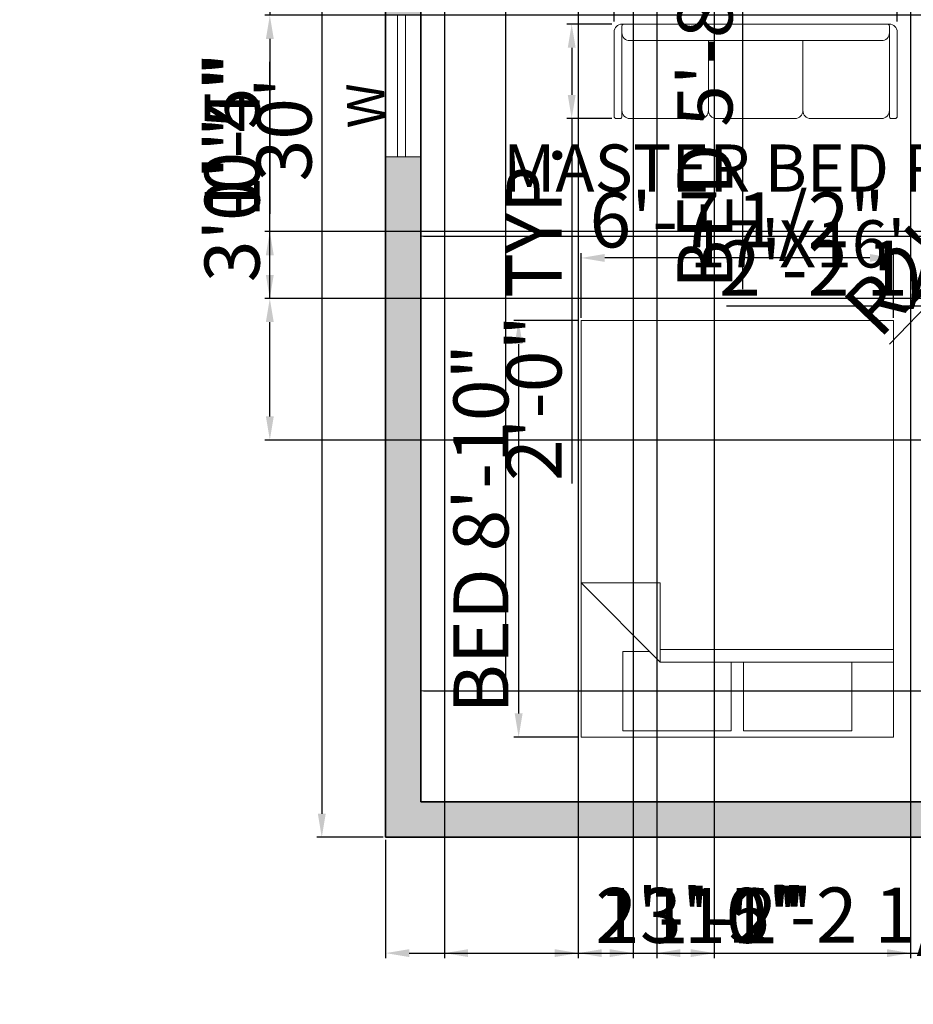
# Model space of a CAD drawing. Units: inches. Extents: x 2961 to 3748, y 1432 to 1961.
# Tile 1 of 9: x 2961 to 3188, y 1462 to 1713. Entities that reach past the tile are written whole.
import ezdxf
from ezdxf.enums import TextEntityAlignment as Align

# ---------------------------------------------------------------- set-up
doc = ezdxf.new("R2010")
doc.units = ezdxf.units.IN
for name, color, linetype, lineweight in [('A-ANNO-DIMS', 2, 'Continuous', 18), ('A-ANNO-TEXT', 7, 'Continuous', 18), ('A-AREA-IDEN', 7, 'Continuous', 18), ('A-FURN', 8, 'Continuous', 18), ('A-FURN-FIXD', 9, 'Continuous', 20), ('A-GLAZ', 4, 'Continuous', 18), ('A-WALL', 7, 'Continuous', 35), ('A-WALL-PATT', 252, 'Continuous', 13)]:
    doc.layers.add(name, color=color, linetype=linetype, lineweight=lineweight)
doc.styles.get("Standard").update_dxf_attribs({"font": 'arial.ttf'})
doc.dimstyles.new('ISO-25', dxfattribs={"dimtxt": 14, "dimasz": 6, "dimexe": 1.25, "dimexo": 0.625, "dimtad": 1, "dimlunit": 3, "dimtxsty": 'Standard', "dimcen": 2.5, "dimadec": 0, "dimazin": 0, "dimtfac": 1, "dimtmove": 0, "dimatfit": 3, "dimfxl": 1, "dimarcsym": 0})

# ---------------------------------------------------------------- blocks, each defined once
blk = doc.blocks.new('Bed - Queen')
for p, q in [((0, -80.00003), (0, 0)), ((0, 0), (59.99999, 0)), ((59.99999, 0), (59.99999, -80.00003)), ((7.99999, -1.2), (28.79998, -1.2)), ((7.99999, -14.4), (7.99999, -1.2)), ((28.79998, -1.2), (28.79998, -14.4)), ((31.19999, -1.2), (51.99999, -1.2)), ((31.19999, -14.4), (31.19999, -1.2)), ((51.99999, -1.2), (51.99999, -16.4)), ((0, -14.4), (44.8, -14.4)), ((59.99999, -29.6), (44.8, -14.4)), ((44.8, -14.4), (44.8, -29.6)), ((44.8, -16.8), (0, -16.8)), ((51.99999, -16.4), (46.79936, -16.4)), ((44.8, -29.6), (59.99999, -29.6)), ((59.99999, -80.00003), (0, -80.00003))]:
    blk.add_line(p, q)
blk = doc.blocks.new('sofa')
for p, q in [((1024.17, 311.16), (1024.17, 289.66)), ((1024.67, 311.66), (1025.67, 311.66)), ((1026.17, 308), (1026.17, 311.16)), ((1050.17, 311.66), (1070.17, 311.66)), ((1094.17, 309.66), (1094.17, 311.16)), ((1095.67, 311.66), (1094.67, 311.66)), ((1096.17, 289.66), (1096.17, 311.16)), ((1048.17, 309.66), (1048.17, 291.87)), ((1048.17, 309.66), (1048.17, 309.66)), ((1072.17, 309.66), (1072.17, 291.87)), ((1072.17, 309.66), (1072.17, 309.66)), ((1026.17, 287.66), (1094.17, 287.66))]:
    blk.add_line(p, q)
for points in [[(1046.17, 311.66), (1028.17, 311.66, 0.414214), (1026.17, 309.66), (1026.17, 288.16)], [(1074.17, 311.66), (1092.17, 311.66, -0.414214), (1094.17, 309.66), (1094.17, 288.16)]]:
    blk.add_lwpolyline(points, format="xyb")
blk.add_lwpolyline([(1026.67, 287.66), (1093.67, 287.66, 0.414214), (1094.17, 288.16), (1094.17, 289.87, 0.414214), (1092.17, 291.87), (1028.17, 291.87, 0.414214), (1026.17, 289.87), (1026.17, 288.16, 0.414214)], format="xyb", close=True)
for centre, radius, start, end in [((1024.67, 311.16), 0.5, 90, 180), ((1025.67, 311.16), 0.5, 0, 90), ((1046.17, 309.66), 2, 0, 90), ((1050.17, 309.66), 2, 90, 180), ((1070.17, 309.66), 2, 0, 90), ((1074.17, 309.66), 2, 90, 180), ((1094.67, 311.16), 0.5, 90, 180), ((1095.67, 311.16), 0.5, 0, 90), ((1026.17, 289.66), 2, 180, 270), ((1094.17, 289.66), 2, 270, 0)]:
    blk.add_arc(centre, radius, start, end)
blk = doc.blocks.new('*D15')
at = {"layer": 'A-ANNO-DIMS', "color": 0, "lineweight": -2, "transparency": 16777216}
for p, q in [((3053.64, 1864.64), (3036.79, 1864.64)), ((3038.04, 1858.64), (3038.04, 1510.64)), ((3053.64, 1504.64), (3036.79, 1504.64))]:
    blk.add_line(p, q, dxfattribs=at)
at = {"layer": 'A-ANNO-DIMS', "color": 0, "transparency": 16777216}
for points in [[(3037.04, 1858.64), (3039.04, 1858.64), (3038.04, 1864.64)], [(3037.04, 1510.64), (3039.04, 1510.64), (3038.04, 1504.64)]]:
    blk.add_solid(points, dxfattribs=at)
at = {"layer": 'Defpoints', "color": 0, "transparency": 16777216}
for p in [(3054.27, 1864.64), (3038.04, 1504.64), (3054.27, 1504.64)]:
    blk.add_point(p, dxfattribs=at)
at = {"layer": 'A-ANNO-DIMS', "color": 0, "transparency": 16777216, "insert": (3030.26, 1684.64), "char_height": 14, "attachment_point": 5, "rotation": 90}
blk.add_mtext("30'", dxfattribs=at)
blk = doc.blocks.new('WIN-36IN')
for p, q in [((0, 6), (36, 6)), ((0, 3.9), (36, 3.9))]:
    blk.add_line(p, q)
blk.add_lwpolyline([(36, 9), (0, 9), (0, 0), (36, 0)], close=True)
blk = doc.blocks.new('*D22')
at = {"layer": 'A-ANNO-DIMS', "color": 0, "lineweight": -2, "transparency": 16777216}
for p, q in [((3103.38, 1636.05), (3086.86, 1636.05)), ((3088.11, 1630.05), (3088.11, 1536.12)), ((3103.38, 1530.12), (3086.86, 1530.12))]:
    blk.add_line(p, q, dxfattribs=at)
at = {"layer": 'A-ANNO-DIMS', "color": 0, "transparency": 16777216}
for points in [[(3087.11, 1630.05), (3089.11, 1630.05), (3088.11, 1636.05)], [(3087.11, 1536.12), (3089.11, 1536.12), (3088.11, 1530.12)]]:
    blk.add_solid(points, dxfattribs=at)
at = {"layer": 'Defpoints', "color": 0, "transparency": 16777216}
for p in [(3104, 1636.05), (3088.11, 1530.12), (3104, 1530.12)]:
    blk.add_point(p, dxfattribs=at)
at = {"layer": 'A-ANNO-DIMS', "color": 0, "transparency": 16777216, "insert": (3080.34, 1583.09), "char_height": 14, "attachment_point": 5, "rotation": 90}
blk.add_mtext('BED 8\'-10"', dxfattribs=at)
blk = doc.blocks.new('*D23')
at = {"layer": 'A-ANNO-DIMS', "color": 0, "lineweight": -2, "transparency": 16777216}
for p, q in [((3104, 1636.67), (3104, 1653.19)), ((3183.44, 1636.67), (3183.44, 1653.19)), ((3177.44, 1651.94), (3110, 1651.94))]:
    blk.add_line(p, q, dxfattribs=at)
at = {"layer": 'A-ANNO-DIMS', "color": 0, "transparency": 16777216}
for points in [[(3110, 1652.94), (3110, 1650.94), (3104, 1651.94)], [(3177.44, 1652.94), (3177.44, 1650.94), (3183.44, 1651.94)]]:
    blk.add_solid(points, dxfattribs=at)
at = {"layer": 'Defpoints', "color": 0, "transparency": 16777216}
for p in [(3104, 1651.94), (3104, 1636.05), (3183.44, 1636.05)]:
    blk.add_point(p, dxfattribs=at)
at = {"layer": 'A-ANNO-DIMS', "color": 0, "transparency": 16777216, "insert": (3143.72, 1659.8), "char_height": 14, "attachment_point": 5}
blk.add_mtext('6\'-7 1/2"', dxfattribs=at)
blk = doc.blocks.new('*D24')
at = {"layer": 'A-ANNO-DIMS', "color": 0, "lineweight": -2, "transparency": 16777216}
for p, q in [((3154.63, 1801.29), (3143.84, 1801.29)), ((3145.09, 1795.29), (3145.09, 1739.5)), ((3154.63, 1733.5), (3143.84, 1733.5)), ((3145.09, 1733.5), (3145.09, 1644.01))]:
    blk.add_line(p, q, dxfattribs=at)
at = {"layer": 'A-ANNO-DIMS', "color": 0, "transparency": 16777216}
for points in [[(3144.09, 1795.29), (3146.09, 1795.29), (3145.09, 1801.29)], [(3144.09, 1739.5), (3146.09, 1739.5), (3145.09, 1733.5)]]:
    blk.add_solid(points, dxfattribs=at)
at = {"layer": 'Defpoints', "color": 0, "transparency": 16777216}
for p in [(3155.26, 1801.29), (3145.09, 1733.5), (3155.26, 1733.5)]:
    blk.add_point(p, dxfattribs=at)
at = {"layer": 'A-ANNO-DIMS', "color": 0, "transparency": 16777216, "insert": (3137.32, 1685.76), "char_height": 14, "attachment_point": 5, "rotation": 90}
blk.add_mtext('BED 5\'-8"', dxfattribs=at)
blk = doc.blocks.new('*D26')
at = {"layer": 'A-ANNO-DIMS', "color": 0, "lineweight": -2, "transparency": 16777216}
for p, q in [((3112.4, 1712.02), (3112.4, 1723.44)), ((3184.4, 1712.02), (3184.4, 1723.44)), ((3112.4, 1722.19), (2961.2, 1722.19)), ((3178.4, 1722.19), (3118.4, 1722.19))]:
    blk.add_line(p, q, dxfattribs=at)
at = {"layer": 'A-ANNO-DIMS', "color": 0, "transparency": 16777216}
for points in [[(3118.4, 1723.19), (3118.4, 1721.19), (3112.4, 1722.19)], [(3178.4, 1723.19), (3178.4, 1721.19), (3184.4, 1722.19)]]:
    blk.add_solid(points, dxfattribs=at)
at = {"layer": 'Defpoints', "color": 0, "transparency": 16777216}
for p in [(3112.4, 1722.19), (3112.4, 1711.39), (3184.4, 1711.39)]:
    blk.add_point(p, dxfattribs=at)
at = {"layer": 'A-ANNO-DIMS', "color": 0, "transparency": 16777216, "insert": (3033.8, 1730.06), "char_height": 14, "attachment_point": 5}
blk.add_mtext('SOFA 6\'-0" TYP.', dxfattribs=at)
blk = doc.blocks.new('*D27')
at = {"layer": 'A-ANNO-DIMS', "color": 0, "lineweight": -2, "transparency": 16777216}
for p, q in [((3111.78, 1711.39), (3100.35, 1711.39)), ((3101.6, 1705.39), (3101.6, 1693.39)), ((3111.78, 1687.39), (3100.35, 1687.39)), ((3101.6, 1687.39), (3101.6, 1594.57))]:
    blk.add_line(p, q, dxfattribs=at)
at = {"layer": 'A-ANNO-DIMS', "color": 0, "transparency": 16777216}
for points in [[(3100.6, 1705.39), (3102.6, 1705.39), (3101.6, 1711.39)], [(3100.6, 1693.39), (3102.6, 1693.39), (3101.6, 1687.39)]]:
    blk.add_solid(points, dxfattribs=at)
at = {"layer": 'Defpoints', "color": 0, "transparency": 16777216}
for p in [(3112.4, 1711.39), (3101.6, 1687.39), (3112.4, 1687.39)]:
    blk.add_point(p, dxfattribs=at)
at = {"layer": 'A-ANNO-DIMS', "color": 0, "transparency": 16777216, "insert": (3093.83, 1637.98), "char_height": 14, "attachment_point": 5, "rotation": 90}
blk.add_mtext('2\'-0" TYP.', dxfattribs=at)
blk = doc.blocks.new('*D29')
at = {"layer": 'A-ANNO-DIMS', "color": 0, "lineweight": -2, "transparency": 16777216}
for p, q in [((3218.32, 1632.29), (3218.32, 1640.93)), ((3245.04, 1632.29), (3245.04, 1640.93)), ((3218.32, 1639.68), (3140.99, 1639.68)), ((3239.04, 1639.68), (3224.32, 1639.68))]:
    blk.add_line(p, q, dxfattribs=at)
at = {"layer": 'A-ANNO-DIMS', "color": 0, "transparency": 16777216}
for points in [[(3224.32, 1640.68), (3224.32, 1638.68), (3218.32, 1639.68)], [(3239.04, 1640.68), (3239.04, 1638.68), (3245.04, 1639.68)]]:
    blk.add_solid(points, dxfattribs=at)
at = {"layer": 'Defpoints', "color": 0, "transparency": 16777216}
for p in [(3218.32, 1639.68), (3218.32, 1631.67), (3245.04, 1631.67)]:
    blk.add_point(p, dxfattribs=at)
at = {"layer": 'A-ANNO-DIMS', "color": 0, "transparency": 16777216, "insert": (3176.66, 1647.55), "char_height": 14, "attachment_point": 5}
blk.add_mtext('2\'-2 1/2"', dxfattribs=at)
blk = doc.blocks.new('*D53')
at = {"layer": 'A-ANNO-DIMS', "color": 0, "lineweight": -2, "transparency": 16777216}
for p, q in [((3123.27, 1855.01), (3123.27, 1473.94)), ((3187.8, 1855.01), (3187.8, 1473.94)), ((3129.27, 1475.19), (3181.8, 1475.19)), ((3187.8, 1475.19), (3264.89, 1475.19))]:
    blk.add_line(p, q, dxfattribs=at)
at = {"layer": 'A-ANNO-DIMS', "color": 0, "transparency": 16777216}
for points in [[(3129.27, 1476.19), (3129.27, 1474.19), (3123.27, 1475.19)], [(3181.8, 1476.19), (3181.8, 1474.19), (3187.8, 1475.19)]]:
    blk.add_solid(points, dxfattribs=at)
at = {"layer": 'Defpoints', "color": 0, "transparency": 16777216}
for p in [(3123.27, 1855.64), (3187.8, 1855.64), (3187.8, 1475.19)]:
    blk.add_point(p, dxfattribs=at)
at = {"layer": 'A-ANNO-DIMS', "color": 0, "transparency": 16777216, "insert": (3229.35, 1483.05), "char_height": 14, "attachment_point": 5}
blk.add_mtext('5\'-4 1/2"', dxfattribs=at)
blk = doc.blocks.new('*D56')
at = {"layer": 'A-ANNO-DIMS', "color": 0, "lineweight": -2, "transparency": 16777216}
for p, q in [((3054.27, 1504.01), (3054.27, 1473.94)), ((3215.27, 1504.01), (3215.27, 1473.94)), ((3060.27, 1475.19), (3209.27, 1475.19))]:
    blk.add_line(p, q, dxfattribs=at)
at = {"layer": 'A-ANNO-DIMS', "color": 0, "transparency": 16777216}
for points in [[(3060.27, 1476.19), (3060.27, 1474.19), (3054.27, 1475.19)], [(3209.27, 1476.19), (3209.27, 1474.19), (3215.27, 1475.19)]]:
    blk.add_solid(points, dxfattribs=at)
at = {"layer": 'Defpoints', "color": 0, "transparency": 16777216}
for p in [(3054.27, 1504.64), (3215.27, 1504.64), (3215.27, 1475.19)]:
    blk.add_point(p, dxfattribs=at)
at = {"layer": 'A-ANNO-DIMS', "color": 0, "transparency": 16777216, "insert": (3134.77, 1482.97), "char_height": 14, "attachment_point": 5}
blk.add_mtext('13\'-5"', dxfattribs=at)
blk = doc.blocks.new('*D68')
at = {"layer": 'A-ANNO-DIMS', "color": 0, "lineweight": -2, "transparency": 16777216}
for p, q in [((3024.82, 1658.64), (3024.82, 1701.79)), ((3509.64, 1658.64), (3023.57, 1658.64)), ((3024.82, 1647.64), (3024.82, 1652.64)), ((3509.64, 1641.64), (3023.57, 1641.64))]:
    blk.add_line(p, q, dxfattribs=at)
at = {"layer": 'A-ANNO-DIMS', "color": 0, "transparency": 16777216}
for points in [[(3023.82, 1652.64), (3025.82, 1652.64), (3024.82, 1658.64)], [(3023.82, 1647.64), (3025.82, 1647.64), (3024.82, 1641.64)]]:
    blk.add_solid(points, dxfattribs=at)
at = {"layer": 'Defpoints', "color": 0, "transparency": 16777216}
for p in [(3024.82, 1658.64), (3510.27, 1658.64), (3510.27, 1641.64)]:
    blk.add_point(p, dxfattribs=at)
at = {"layer": 'A-ANNO-DIMS', "color": 0, "transparency": 16777216, "insert": (3017.04, 1683.21), "char_height": 14, "attachment_point": 5, "rotation": 90}
blk.add_mtext('1\'-5"', dxfattribs=at)
blk = doc.blocks.new('*D70')
at = {"layer": 'A-ANNO-DIMS', "color": 0, "lineweight": -2, "transparency": 16777216}
for p, q in [((3024.82, 1641.64), (3024.82, 1686.09)), ((3383.64, 1641.64), (3023.57, 1641.64)), ((3024.82, 1611.64), (3024.82, 1635.64)), ((3383.64, 1605.64), (3023.57, 1605.64))]:
    blk.add_line(p, q, dxfattribs=at)
at = {"layer": 'A-ANNO-DIMS', "color": 0, "transparency": 16777216}
for points in [[(3023.82, 1635.64), (3025.82, 1635.64), (3024.82, 1641.64)], [(3023.82, 1611.64), (3025.82, 1611.64), (3024.82, 1605.64)]]:
    blk.add_solid(points, dxfattribs=at)
at = {"layer": 'Defpoints', "color": 0, "transparency": 16777216}
for p in [(3024.82, 1641.64), (3384.27, 1641.64), (3384.27, 1605.64)]:
    blk.add_point(p, dxfattribs=at)
at = {"layer": 'A-ANNO-DIMS', "color": 0, "transparency": 16777216, "insert": (3017.04, 1666.87), "char_height": 14, "attachment_point": 5, "rotation": 90}
blk.add_mtext('3\'-0"', dxfattribs=at)
blk = doc.blocks.new('*D73')
at = {"layer": 'A-ANNO-DIMS', "color": 0, "lineweight": -2, "transparency": 16777216}
for p, q in [((3069.27, 1717.01), (3069.27, 1473.94)), ((3103.27, 1717.01), (3103.27, 1473.94)), ((3075.27, 1475.19), (3097.27, 1475.19)), ((3103.27, 1475.19), (3158.85, 1475.19))]:
    blk.add_line(p, q, dxfattribs=at)
at = {"layer": 'A-ANNO-DIMS', "color": 0, "transparency": 16777216}
for points in [[(3075.27, 1476.19), (3075.27, 1474.19), (3069.27, 1475.19)], [(3097.27, 1476.19), (3097.27, 1474.19), (3103.27, 1475.19)]]:
    blk.add_solid(points, dxfattribs=at)
at = {"layer": 'Defpoints', "color": 0, "transparency": 16777216}
for p in [(3069.27, 1717.64), (3103.27, 1717.64), (3103.27, 1475.19)]:
    blk.add_point(p, dxfattribs=at)
at = {"layer": 'A-ANNO-DIMS', "color": 0, "transparency": 16777216, "insert": (3134.06, 1482.96), "char_height": 14, "attachment_point": 5}
blk.add_mtext('2\'-10"', dxfattribs=at)
blk = doc.blocks.new('*D74')
at = {"layer": 'A-ANNO-DIMS', "color": 0, "lineweight": -2, "transparency": 16777216}
for p, q in [((3117.27, 1726.01), (3117.27, 1473.94)), ((3103.27, 1717.01), (3103.27, 1473.94)), ((3109.27, 1475.19), (3111.27, 1475.19)), ((3117.27, 1475.19), (3160.41, 1475.19))]:
    blk.add_line(p, q, dxfattribs=at)
at = {"layer": 'A-ANNO-DIMS', "color": 0, "transparency": 16777216}
for points in [[(3109.27, 1476.19), (3109.27, 1474.19), (3103.27, 1475.19)], [(3111.27, 1476.19), (3111.27, 1474.19), (3117.27, 1475.19)]]:
    blk.add_solid(points, dxfattribs=at)
at = {"layer": 'Defpoints', "color": 0, "transparency": 16777216}
for p in [(3117.27, 1726.64), (3103.27, 1717.64), (3117.27, 1475.19)]:
    blk.add_point(p, dxfattribs=at)
at = {"layer": 'A-ANNO-DIMS', "color": 0, "transparency": 16777216, "insert": (3141.84, 1482.84), "char_height": 14, "attachment_point": 5}
blk.add_mtext('1\'-2"', dxfattribs=at)
blk = doc.blocks.new('*D75')
at = {"layer": 'A-ANNO-DIMS', "color": 0, "lineweight": -2, "transparency": 16777216}
for p, q in [((3024.82, 1723.64), (3024.82, 1729.64)), ((3254.64, 1717.64), (3023.57, 1717.64)), ((3024.82, 1717.64), (3024.82, 1713.64)), ((3254.64, 1713.64), (3023.57, 1713.64)), ((3024.82, 1707.64), (3024.82, 1663.17))]:
    blk.add_line(p, q, dxfattribs=at)
at = {"layer": 'A-ANNO-DIMS', "color": 0, "transparency": 16777216}
for points in [[(3023.82, 1723.64), (3025.82, 1723.64), (3024.82, 1717.64)], [(3023.82, 1707.64), (3025.82, 1707.64), (3024.82, 1713.64)]]:
    blk.add_solid(points, dxfattribs=at)
at = {"layer": 'Defpoints', "color": 0, "transparency": 16777216}
for p in [(3255.27, 1717.64), (3024.82, 1713.64), (3255.27, 1713.64)]:
    blk.add_point(p, dxfattribs=at)
at = {"layer": 'A-ANNO-DIMS', "color": 0, "transparency": 16777216, "insert": (3017.04, 1682.41), "char_height": 14, "attachment_point": 5, "rotation": 90}
blk.add_mtext('0\'-4"', dxfattribs=at)
blk = doc.blocks.new('*D81')
at = {"layer": 'A-ANNO-DIMS', "color": 0, "lineweight": -2, "transparency": 16777216}
for p, q in [((3063.89, 1657.48), (3633.97, 1657.48)), ((3632.72, 1547.87), (3632.72, 1651.48)), ((3063.89, 1541.87), (3633.97, 1541.87))]:
    blk.add_line(p, q, dxfattribs=at)
at = {"layer": 'A-ANNO-DIMS', "color": 0, "transparency": 16777216}
for points in [[(3631.72, 1651.48), (3633.72, 1651.48), (3632.72, 1657.48)], [(3631.72, 1547.87), (3633.72, 1547.87), (3632.72, 1541.87)]]:
    blk.add_solid(points, dxfattribs=at)
at = {"layer": 'Defpoints', "color": 0, "transparency": 16777216}
for p in [(3063.27, 1657.48), (3632.72, 1657.48), (3063.27, 1541.87)]:
    blk.add_point(p, dxfattribs=at)
at = {"layer": 'A-ANNO-DIMS', "color": 0, "transparency": 16777216, "insert": (3624.85, 1599.67), "char_height": 14, "attachment_point": 5, "rotation": 90}
blk.add_mtext('9\'-7 1/2"', dxfattribs=at)
blk = doc.blocks.new('*D82')
at = {"layer": 'A-ANNO-DIMS', "color": 0, "lineweight": -2, "transparency": 16777216}
for p, q in [((3063.27, 1542.49), (3063.27, 1933.63)), ((3084.82, 1542.49), (3084.82, 1933.63)), ((3069.27, 1932.38), (3078.82, 1932.38)), ((3084.82, 1932.38), (3160.59, 1932.38))]:
    blk.add_line(p, q, dxfattribs=at)
at = {"layer": 'A-ANNO-DIMS', "color": 0, "transparency": 16777216}
for points in [[(3069.27, 1933.38), (3069.27, 1931.38), (3063.27, 1932.38)], [(3078.82, 1933.38), (3078.82, 1931.38), (3084.82, 1932.38)]]:
    blk.add_solid(points, dxfattribs=at)
at = {"layer": 'Defpoints', "color": 0, "transparency": 16777216}
for p in [(3084.82, 1932.38), (3063.27, 1541.87), (3084.82, 1541.87)]:
    blk.add_point(p, dxfattribs=at)
at = {"layer": 'A-ANNO-DIMS', "color": 0, "transparency": 16777216, "insert": (3125.71, 1940.24), "char_height": 14, "attachment_point": 5}
blk.add_mtext('1\'-9 1/2"', dxfattribs=at)
blk = doc.blocks.new('*D84')
at = {"layer": 'A-ANNO-DIMS', "color": 0, "lineweight": -2, "transparency": 16777216}
for p, q in [((3123.27, 1855.01), (3123.27, 1473.94)), ((3137.88, 1855.01), (3137.88, 1473.94)), ((3129.27, 1475.19), (3131.88, 1475.19)), ((3137.88, 1475.19), (3213.65, 1475.19))]:
    blk.add_line(p, q, dxfattribs=at)
at = {"layer": 'A-ANNO-DIMS', "color": 0, "transparency": 16777216}
for points in [[(3129.27, 1476.19), (3129.27, 1474.19), (3123.27, 1475.19)], [(3131.88, 1476.19), (3131.88, 1474.19), (3137.88, 1475.19)]]:
    blk.add_solid(points, dxfattribs=at)
at = {"layer": 'Defpoints', "color": 0, "transparency": 16777216}
for p in [(3123.27, 1855.64), (3137.88, 1855.64), (3137.88, 1475.19)]:
    blk.add_point(p, dxfattribs=at)
at = {"layer": 'A-ANNO-DIMS', "color": 0, "transparency": 16777216, "insert": (3178.76, 1483.05), "char_height": 14, "attachment_point": 5}
blk.add_mtext('1\'-2 1/2"', dxfattribs=at)
blk = doc.blocks.new('*D93')
at = {"layer": 'A-ANNO-DIMS', "color": 0, "lineweight": -2, "transparency": 16777216}
for p, q in [((3257.58, 1708.39), (3234.18, 1683.97)), ((3182.46, 1630.01), (3230.03, 1679.64))]:
    blk.add_line(p, q, dxfattribs=at)
at = {"layer": 'A-ANNO-DIMS', "color": 0, "transparency": 16777216}
blk.add_solid([(3229.31, 1680.33), (3230.75, 1678.95), (3234.18, 1683.97)], dxfattribs=at)
at = {"layer": 'Defpoints', "color": 0, "transparency": 16777216}
for p in [(3257.58, 1708.39), (3234.18, 1683.97)]:
    blk.add_point(p, dxfattribs=at)
at = {"layer": 'A-ANNO-DIMS', "color": 0, "transparency": 16777216, "insert": (3198.56, 1658.04), "char_height": 14, "attachment_point": 5, "rotation": 46.2188}
blk.add_mtext('R2\'-10"', dxfattribs=at)

msp = doc.modelspace()

# ---------------------------------------------------------------- hatches: boundary and pattern name
at = {"layer": 'A-WALL-PATT'}
h = msp.add_hatch(color=256, dxfattribs=at)
h.set_gradient(color1=(41, 49, 137), color2=(41, 49, 137), tint=1)
h.paths.add_polyline_path([(3255.267, 1671.639), (3255.267, 1513.639), (3251.267, 1513.639), (3251.267, 1504.639), (3268.267, 1504.639), (3268.267, 1513.639), (3264.267, 1513.639), (3264.267, 1671.639), (3259.767, 1671.639)])
h.paths.add_polyline_path([(3063.267, 1513.639), (3063.267, 1677.639), (3054.267, 1677.639), (3054.267, 1504.639), (3215.267, 1504.639), (3215.267, 1513.639)])
h.paths.add_polyline_path([(3304.267, 1513.639), (3304.267, 1504.639), (3456.267, 1504.639), (3456.267, 1513.639), (3390.267, 1513.639), (3390.267, 1605.639), (3384.267, 1605.639), (3384.267, 1513.639)])
h.paths.add_polyline_path([(3510.267, 1605.639), (3510.267, 1513.639), (3492.267, 1513.639), (3492.267, 1504.639), (3546.267, 1504.639), (3546.267, 1513.639), (3519.267, 1513.639), (3519.267, 1605.639)])
h.paths.add_polyline_path([(3340.267, 1654.639), (3340.267, 1645.639), (3510.267, 1645.639), (3510.267, 1641.639), (3519.267, 1641.639), (3519.267, 1658.639), (3510.267, 1658.639), (3510.267, 1654.639)])
h.paths.add_polyline_path([(3223.801, 1864.639), (3223.801, 1855.639), (3255.267, 1855.639), (3255.267, 1772.534), (3264.267, 1772.534), (3264.267, 1855.639), (3303.267, 1855.639), (3303.267, 1864.639)])
h.paths.add_polyline_path([(3339.267, 1864.639), (3339.267, 1855.639), (3435.267, 1855.639), (3435.267, 1864.639)])
h.paths.add_polyline_path([(3471.267, 1864.639), (3471.267, 1855.639), (3510.267, 1855.639), (3510.267, 1827.639), (3519.267, 1827.639), (3519.267, 1864.639)])
h.paths.add_polyline_path([(3510.267, 1767.639), (3510.267, 1739.639), (3519.267, 1739.639), (3519.267, 1767.639)])
h.paths.add_polyline_path([(3123.267, 1726.639), (3123.267, 1855.639), (3187.801, 1855.639), (3187.801, 1864.639), (3054.267, 1864.639), (3054.267, 1837.201), (3063.267, 1837.201), (3063.267, 1855.639), (3117.267, 1855.639), (3117.267, 1726.639), (3103.267, 1726.639), (3103.267, 1717.639), (3255.267, 1717.639), (3255.267, 1713.639), (3264.267, 1713.639), (3264.267, 1730.534), (3255.267, 1730.639), (3255.267, 1726.639)])
h.paths.add_polyline_path([(3597.267, 1654.639), (3597.267, 1513.639), (3570.267, 1513.639), (3570.267, 1504.639), (3603.267, 1504.639), (3603.267, 1654.639)])
h.paths.add_polyline_path([(3054.267, 1813.201), (3054.267, 1713.639), (3063.267, 1713.639), (3063.267, 1717.639), (3069.267, 1717.639), (3069.267, 1726.639), (3063.267, 1726.639), (3063.267, 1813.201)], flags=17)

# ---------------------------------------------------------------- linework, layer by layer
at = {"layer": 'A-FURN-FIXD'}
msp.add_lwpolyline([(3063.267, 1541.867), (3063.267, 1657.476), (3084.825, 1657.476), (3084.825, 1541.867)], close=True, dxfattribs=at)
at = {"layer": 'A-WALL'}
for p, q in [((3054.267, 1504.639), (3054.267, 1864.639)), ((3063.267, 1513.639), (3063.267, 1717.639)), ((3255.267, 1513.639), (3063.267, 1513.639)), ((3603.267, 1504.639), (3054.267, 1504.639))]:
    msp.add_line(p, q, dxfattribs=at)

# ---------------------------------------------------------------- block references
at = {"layer": 'A-FURN', "rotation": 180}
msp.add_blockref('sofa', (4208.569, 1999.053), dxfattribs=at)
at = {"layer": 'A-FURN', "xscale": 1.324028879948369, "yscale": 1.324028879948369, "zscale": 1.324028879948369, "rotation": 180}
msp.add_blockref('Bed - Queen', (3183.443, 1530.125), dxfattribs=at)
at = {"layer": 'A-GLAZ', "rotation": 90.00000000000213}
msp.add_blockref('WIN-36IN', (3063.267, 1677.639), dxfattribs=at)

# ---------------------------------------------------------------- texts
at = {"layer": 'A-ANNO-TEXT'}
msp.add_text('W', height=9.571, rotation=92.15165, dxfattribs=at).set_placement((3054.03, 1690.944), align=Align.CENTER)
at = {"layer": 'A-AREA-IDEN'}
for s, p in [('MASTER BED ROOM', (3159.071, 1668.787)), ("17'X16'", (3159.071, 1649.511))]:
    msp.add_text(s, height=12, dxfattribs=at).set_placement(p, align=Align.CENTER)

# ---------------------------------------------------------------- dimensions: what is measured, and where the dimension line sits
at = {"layer": 'A-ANNO-DIMS'}
for base, p1, p2, picture, middle in [((3084.825, 1932.38), (3063.267, 1541.867), (3084.825, 1541.867), '*D82', (3125.71, 1940.244)), ((3187.801, 1475.189), (3123.267, 1855.639), (3187.801, 1855.639), '*D53', (3229.345, 1483.052)), ((3137.877, 1475.189), (3123.267, 1855.639), (3137.877, 1855.639), '*D84', (3178.762, 1483.052)), ((3117.267, 1475.189), (3103.267, 1717.639), (3117.267, 1726.639), '*D74', (3141.841, 1482.842)), ((3103.267, 1475.189), (3069.267, 1717.639), (3103.267, 1717.639), '*D73', (3134.058, 1482.962)), ((3215.267, 1475.189), (3054.267, 1504.639), (3215.267, 1504.639), '*D56', (3134.767, 1482.966))]:
    dim = msp.add_linear_dim(base=base, p1=p1, p2=p2, dimstyle='ISO-25', override={"dimdec": 1, "dimlfac": 1, "dimrnd": 0, "dimzin": 1, "dimdsep": 46, "dimlunit": 4, "dimfrac": 2}, dxfattribs=at)
    dim.commit()
    dim.dimension.update_dxf_attribs({"geometry": picture, "text_midpoint": middle})
for base, p1, p2, angle, override, picture, middle in [((3038.036, 1504.639), (3054.267, 1864.639), (3054.267, 1504.639), 90, {"dimclrd": 0, "dimclre": 0, "dimclrt": 0}, '*D15', (3030.258, 1684.639)), ((3024.817, 1713.639), (3255.267, 1717.639), (3255.267, 1713.639), 90, {"dimdec": 1, "dimlfac": 1, "dimrnd": 0, "dimzin": 1, "dimdsep": 46, "dimlunit": 4, "dimfrac": 2}, '*D75', (3017.044, 1682.406)), ((3024.817, 1658.639), (3510.267, 1641.639), (3510.267, 1658.639), 90, {"dimdec": 1, "dimlfac": 1, "dimrnd": 0, "dimzin": 1, "dimdsep": 46, "dimlunit": 4, "dimfrac": 2}, '*D68', (3017.044, 1683.212)), ((3024.817, 1641.639), (3384.267, 1605.639), (3384.267, 1641.639), 90, {"dimdec": 1, "dimlfac": 1, "dimrnd": 0, "dimzin": 1, "dimdsep": 46, "dimlunit": 4, "dimfrac": 2}, '*D70', (3017.039, 1666.867)), ((3104.001, 1651.936), (3183.443, 1636.047), (3104.001, 1636.047), 180, {"dimdec": 1, "dimlfac": 1, "dimrnd": 0, "dimzin": 1, "dimdsep": 46, "dimlunit": 4, "dimfrac": 2}, '*D23', (3143.722, 1659.799)), ((3218.321, 1639.684), (3245.042, 1631.667), (3218.321, 1631.667), 180, {"dimdec": 1, "dimlfac": 1, "dimrnd": 0, "dimzin": 1, "dimdsep": 46, "dimlunit": 4, "dimfrac": 2}, '*D29', (3176.657, 1647.547)), ((3632.717, 1657.476), (3063.267, 1541.867), (3063.267, 1657.476), 90, {"dimdec": 1, "dimlfac": 1, "dimrnd": 0, "dimzin": 1, "dimdsep": 46, "dimlunit": 4, "dimfrac": 2}, '*D81', (3624.853, 1599.671))]:
    dim = msp.add_linear_dim(base=base, p1=p1, p2=p2, angle=angle, dimstyle='ISO-25', override=override, dxfattribs=at)
    dim.commit()
    dim.dimension.update_dxf_attribs({"geometry": picture, "text_midpoint": middle})
for base, p1, p2, angle, text, picture, middle in [((3145.088, 1733.502), (3155.257, 1801.293), (3155.257, 1733.502), 270, 'BED <>', '*D24', (3137.315, 1685.756)), ((3112.401, 1722.191), (3184.401, 1711.391), (3112.401, 1711.391), 180, 'SOFA <> TYP.', '*D26', (3033.799, 1730.06)), ((3101.601, 1687.391), (3112.401, 1711.391), (3112.401, 1687.391), 270, '<> TYP.', '*D27', (3093.828, 1637.979)), ((3088.113, 1530.125), (3104.001, 1636.047), (3104.001, 1530.125), 270, 'BED <>', '*D22', (3080.34, 1583.086))]:
    dim = msp.add_linear_dim(base=base, p1=p1, p2=p2, angle=angle, text=text, dimstyle='ISO-25', override={"dimdec": 1, "dimlfac": 1, "dimrnd": 0, "dimzin": 1, "dimdsep": 46, "dimlunit": 4, "dimfrac": 2}, dxfattribs=at)
    dim.commit()
    dim.dimension.update_dxf_attribs({"geometry": picture, "text_midpoint": middle})
dim = msp.add_radius_dim(center=(3257.579, 1708.389), mpoint=(3234.178, 1683.97), dimstyle='ISO-25', override={"dimdec": 1, "dimlfac": 1, "dimrnd": 0, "dimzin": 1, "dimdsep": 46, "dimlunit": 4, "dimfrac": 2}, dxfattribs=at)
dim.commit()
dim.dimension.update_dxf_attribs({"geometry": '*D93', "text_midpoint": (3198.558, 1658.036)})

doc.saveas('drawing.dxf')
